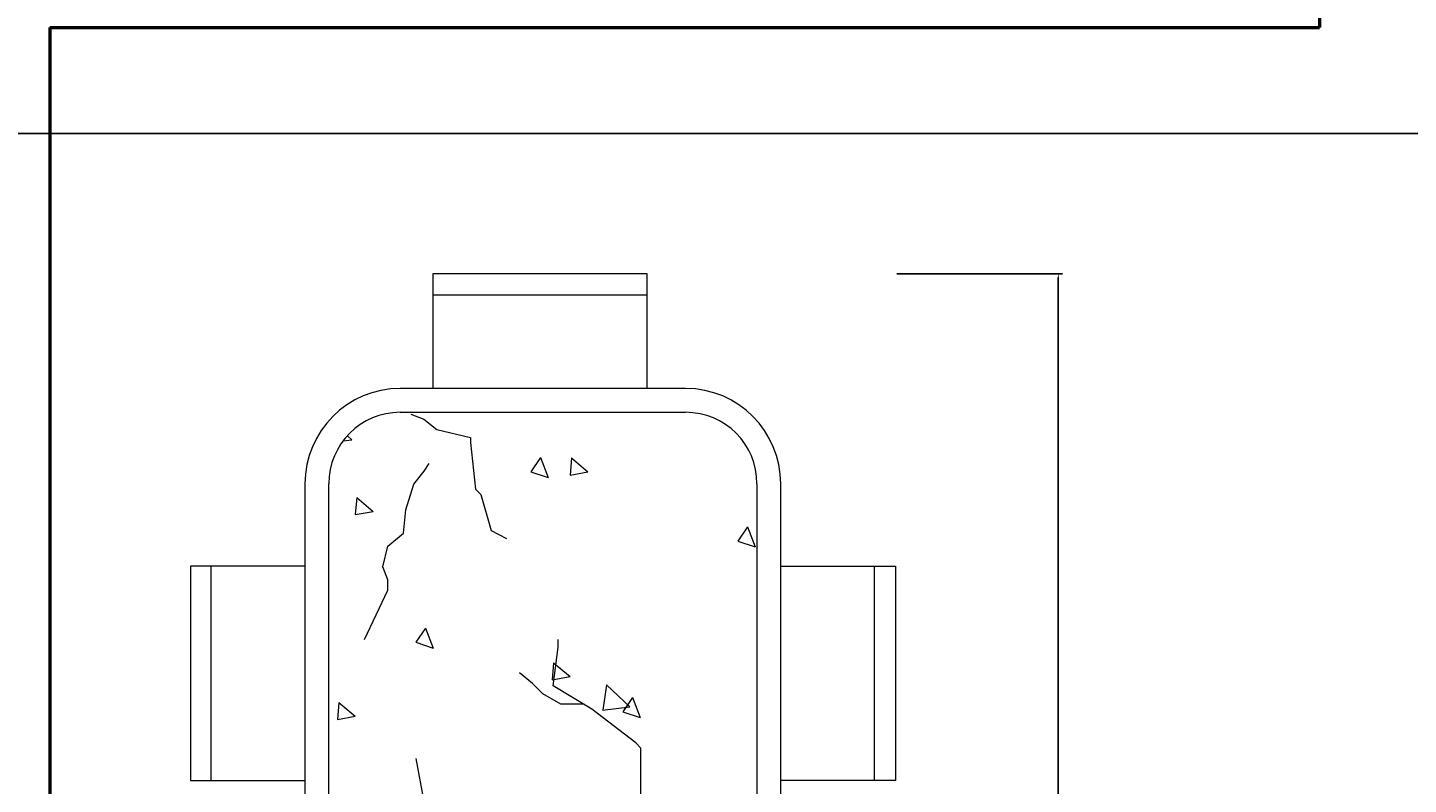
# Model space of a CAD drawing. Units: inches. Extents: x -173 to 545, y -746 to 104.
# Tile 18 of 32: x 314 to 373, y -496 to -463. Entities that reach past the tile are written whole.
import ezdxf

# ---------------------------------------------------------------- set-up
doc = ezdxf.new("R2010")
doc.units = ezdxf.units.IN
doc.header["$MEASUREMENT"] = 0
for name, color, linetype, lineweight in [('A-ANNO-DIMS', 2, 'Continuous', 18), ('A-FURN', 8, 'Continuous', 18), ('A-WALL', 7, 'Continuous', 50)]:
    doc.layers.add(name, color=color, linetype=linetype, lineweight=lineweight)
doc.styles.get("Standard").update_dxf_attribs({"font": 'arial.ttf'})
doc.dimstyles.get("Standard").update_dxf_attribs({"dimtxt": 0.18, "dimasz": 0.18, "dimexe": 0.18, "dimexo": 0.0625, "dimgap": 0.09, "dimtad": 0, "dimtih": 1, "dimtoh": 1, "dimdec": 0, "dimzin": 0, "dimdsep": 46, "dimlunit": 3, "dimtxsty": 'Standard', "dimcen": 0.09, "dimadec": 0, "dimazin": 0, "dimtfac": 1, "dimtdec": 0, "dimtofl": 0, "dimtmove": 0, "dimatfit": 3, "dimfxl": 1, "dimtolj": 1, "dimtzin": 0, "dimarcsym": 0})

# ---------------------------------------------------------------- blocks, each defined once
blk = doc.blocks.new('DINING-TABLE-SIX')
for p, q in [((19.425, 46.174), (10.319, 46.174)), ((10.319, 46.174), (10.319, 41.298)), ((19.425, 41.298), (19.425, 46.174)), ((10.319, 45.284), (19.425, 45.284)), ((21.064, 41.298), (8.923, 41.298)), ((8.923, 40.286), (21.064, 40.286)), ((9.384, 40.21), (9.934, 39.99)), ((9.934, 39.99), (10.483, 39.549)), ((10.483, 39.549), (11.912, 39.219)), ((6.494, 39.071), (6.862, 39.113)), ((6.677, 39.292), (6.862, 39.113)), ((11.912, 39.219), (11.912, 38.999)), ((11.912, 38.999), (12.132, 37.019)), ((14.891, 38.367), (14.483, 37.763)), ((14.891, 38.367), (15.217, 37.517)), ((16.212, 38.347), (16.148, 37.621)), ((16.212, 38.347), (16.909, 37.762)), ((9.498, 37.238), (9.938, 37.788)), ((9.938, 37.788), (10.158, 38.118)), ((14.483, 37.763), (15.217, 37.517)), ((16.148, 37.621), (16.909, 37.762)), ((4.876, 37.251), (4.876, 8.923)), ((5.888, 8.923), (5.888, 37.251)), ((9.169, 36.138), (9.498, 37.238)), ((12.132, 37.019), (12.351, 36.799)), ((24.099, 37.251), (24.099, 8.923)), ((25.11, 8.923), (25.11, 37.251)), ((7.08, 36.662), (7.016, 35.937)), ((7.08, 36.662), (7.777, 36.077)), ((12.351, 36.799), (12.791, 35.259)), ((7.016, 35.937), (7.777, 36.077)), ((9.059, 35.148), (9.169, 36.138)), ((12.791, 35.259), (13.45, 34.929)), ((23.694, 35.413), (23.287, 34.809)), ((23.694, 35.413), (24.021, 34.563)), ((8.4, 34.597), (9.059, 35.148)), ((23.287, 34.809), (24.02, 34.563)), ((8.18, 33.717), (8.4, 34.597)), ((4.876, 33.75), (0, 33.75)), ((0, 33.75), (0, 24.645)), ((0.89, 24.645), (0.89, 33.75)), ((8.4, 33.167), (8.18, 33.717)), ((25.11, 33.75), (29.987, 33.75)), ((29.097, 24.645), (29.097, 33.75)), ((29.987, 33.75), (29.987, 24.645)), ((8.4, 32.727), (8.4, 33.167)), ((7.411, 30.637), (8.4, 32.727)), ((10.003, 31.12), (9.595, 30.516)), ((10.003, 31.12), (10.329, 30.27)), ((15.648, 30.309), (15.648, 30.639)), ((9.595, 30.516), (10.329, 30.27)), ((15.428, 28.659), (15.648, 30.309)), ((15.45, 29.639), (15.387, 28.913)), ((15.45, 29.639), (16.148, 29.054)), ((14.549, 28.769), (14, 29.209)), ((15.386, 28.913), (16.147, 29.054)), ((14.988, 28.329), (14.549, 28.769)), ((15.758, 27.888), (14.988, 28.329)), ((17.076, 27.668), (15.428, 28.659)), ((17.703, 28.712), (17.536, 27.632)), ((17.703, 28.712), (18.689, 27.766)), ((6.318, 27.954), (6.255, 27.229)), ((6.318, 27.954), (7.016, 27.369)), ((16.747, 27.888), (15.758, 27.888)), ((18.944, 26.238), (17.076, 27.668)), ((17.535, 27.632), (18.688, 27.766)), ((18.806, 28.166), (18.399, 27.562)), ((18.806, 28.166), (19.133, 27.316)), ((6.254, 27.229), (7.015, 27.369)), ((18.399, 27.562), (19.132, 27.316)), ((19.164, 26.018), (18.944, 26.238)), ((19.164, 19.638), (19.164, 26.018)), ((9.934, 23.818), (9.604, 25.578)), ((0, 24.645), (4.876, 24.645)), ((29.987, 24.645), (25.11, 24.645))]:
    blk.add_line(p, q)
for centre, radius, start, end in [((8.923, 37.251), 4.047, 90, 180), ((21.064, 37.251), 4.047, 0, 90), ((8.923, 37.251), 3.035, 90, 180), ((21.064, 37.251), 3.035, 0, 90)]:
    blk.add_arc(centre, radius, start, end)
blk = doc.blocks.new('*D52')
at = {"layer": 'A-ANNO-DIMS', "color": 0, "lineweight": -2, "transparency": 16777216}
for p, q in [((351.326, -473.821), (358.369, -473.821)), ((358.189, -474.001), (358.189, -496.725)), ((358.189, -519.816), (358.189, -497.091)), ((351.326, -519.996), (358.369, -519.996))]:
    blk.add_line(p, q, dxfattribs=at)
at = {"layer": 'A-ANNO-DIMS', "color": 0, "transparency": 16777216}
for points in [[(358.159, -474.001), (358.219, -474.001), (358.189, -473.821)], [(358.159, -519.816), (358.219, -519.816), (358.189, -519.996)]]:
    blk.add_solid(points, dxfattribs=at)
at = {"layer": 'Defpoints', "color": 0, "transparency": 16777216}
for p in [(351.263, -473.821), (358.189, -473.821), (351.263, -519.996)]:
    blk.add_point(p, dxfattribs=at)
at = {"layer": 'A-ANNO-DIMS', "color": 0, "transparency": 16777216, "insert": (358.189, -496.908), "char_height": 0.18, "attachment_point": 5}
blk.add_mtext('\\A1;DINING SET 3\'-10" TYP.', dxfattribs=at)
blk = doc.blocks.new('*D82')
at = {"layer": 'A-ANNO-DIMS', "color": 0, "lineweight": -2, "transparency": 16777216}
for p, q in [((219.864, -467.862), (545.081, -467.862)), ((544.901, -468.042), (544.901, -509.68)), ((544.901, -551.682), (544.901, -510.044)), ((219.864, -551.862), (545.081, -551.862))]:
    blk.add_line(p, q, dxfattribs=at)
at = {"layer": 'A-ANNO-DIMS', "color": 0, "transparency": 16777216}
for points in [[(544.871, -468.042), (544.931, -468.042), (544.901, -467.862)], [(544.871, -551.682), (544.931, -551.682), (544.901, -551.862)]]:
    blk.add_solid(points, dxfattribs=at)
at = {"layer": 'Defpoints', "color": 0, "transparency": 16777216}
for p in [(219.801, -467.862), (219.801, -551.862), (544.901, -551.862)]:
    blk.add_point(p, dxfattribs=at)
at = {"layer": 'A-ANNO-DIMS', "color": 0, "transparency": 16777216, "insert": (544.901, -509.862), "char_height": 0.18, "attachment_point": 5}
blk.add_mtext('\\A1;7\'-0"', dxfattribs=at)

msp = doc.modelspace()

# ---------------------------------------------------------------- linework, layer by layer
at = {"layer": 'A-WALL'}
for p, q in [((369.301, -458.862), (369.301, -463.362)), ((315.301, -463.362), (369.301, -463.362)), ((315.301, -463.362), (315.301, -560.862))]:
    msp.add_line(p, q, dxfattribs=at)

# ---------------------------------------------------------------- block references
at = {"layer": 'A-FURN'}
msp.add_blockref('DINING-TABLE-SIX', (321.276, -519.995), dxfattribs=at)

# ---------------------------------------------------------------- dimensions: what is measured, and where the dimension line sits
at = {"layer": 'A-ANNO-DIMS'}
dim = msp.add_linear_dim(base=(544.901, -551.862), p1=(219.801, -467.862), p2=(219.801, -551.862), angle=90, dimstyle='Standard', override={"dimdec": 1, "dimlfac": 1, "dimrnd": 0, "dimzin": 1, "dimdsep": 46, "dimlunit": 4, "dimfrac": 2}, dxfattribs=at)
dim.commit()
dim.dimension.update_dxf_attribs({"geometry": '*D82', "text_midpoint": (544.901, -509.862)})
dim = msp.add_linear_dim(base=(358.189, -473.821), p1=(351.263, -519.996), p2=(351.263, -473.821), angle=90, text='DINING SET <> TYP.', dimstyle='Standard', override={"dimdec": 1, "dimlfac": 1, "dimrnd": 0, "dimzin": 1, "dimdsep": 46, "dimlunit": 4, "dimfrac": 2}, dxfattribs=at)
dim.commit()
dim.dimension.update_dxf_attribs({"geometry": '*D52', "text_midpoint": (358.189, -496.908)})

doc.saveas('drawing.dxf')
